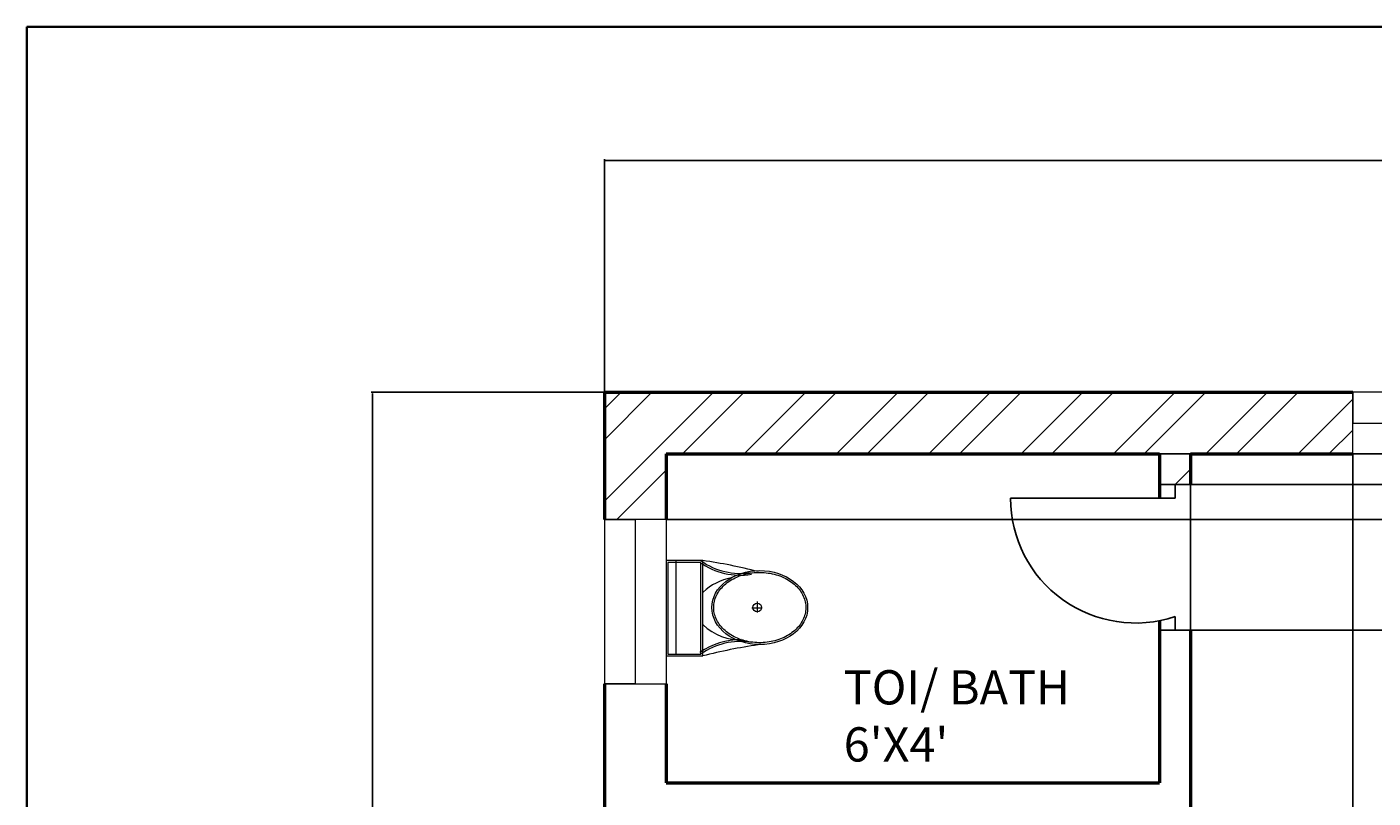
# Model space of a CAD drawing. Units: inches. Extents: x 2310 to 2937, y 1113 to 2410.
# Tile 18 of 23: x 2310 to 2507, y 2297 to 2410. Entities that reach past the tile are written whole.
import ezdxf

# ---------------------------------------------------------------- set-up
doc = ezdxf.new("R2010")
doc.units = ezdxf.units.IN
for name, color, linetype, lineweight in [('A-ANNO-DIMS', 2, 'Continuous', 18), ('A-ANNO-TTLB', 7, 'Continuous', 35), ('A-AREA-IDEN', 7, 'Continuous', 18), ('A-DOOR', 31, 'Continuous', 25), ('A-FLOR-FIXT', 9, 'Continuous', 18), ('A-GLAZ', 191, 'Continuous', 20), ('A-WALL', 7, 'Continuous', 50), ('A-WALL-PATT', 85, 'Continuous', 13)]:
    doc.layers.add(name, color=color, linetype=linetype, lineweight=lineweight)
doc.styles.get("Standard").update_dxf_attribs({"font": 'arial.ttf'})
doc.dimstyles.get("Standard").update_dxf_attribs({"dimtxt": 0.18, "dimasz": 0.18, "dimexe": 0.18, "dimexo": 0.0625, "dimgap": 0.09, "dimtad": 0, "dimtih": 1, "dimtoh": 1, "dimdec": 4, "dimzin": 0, "dimdsep": 46, "dimtxsty": 'Standard', "dimcen": 0.09, "dimadec": 0, "dimazin": 0, "dimtfac": 1, "dimtdec": 4, "dimtofl": 0, "dimtmove": 0, "dimatfit": 3, "dimfxl": 1, "dimtolj": 1, "dimtzin": 0, "dimarcsym": 0})

# ---------------------------------------------------------------- blocks, each defined once
blk = doc.blocks.new('A$C31115884')
for p, q in [((257.5, 466.4), (257.5, 523.2)), ((283.1, 497.7), (223.4, 497.7)), ((0, 200), (0, 0)), ((520, 200), (0, 200)), ((10, 190), (10, 10)), ((510, 190), (10, 190)), ((510, 10), (510, 190)), ((520, 0), (520, 200)), ((510, 54.5), (0, 54.5)), ((10, 10), (510, 10)), ((0, 0), (520, 0))]:
    blk.add_line(p, q)
blk.add_circle((255.6, 496.4), 23.6)
for centre, radius, start, end in [((2777.7, -204.6), 2807, 165.4549, 171.71327), ((-294.5, 403.3), 364.7, 324.20913, 9.34987), ((-294.5, 403.3), 374.7, 324.20913, 9.34987), ((805.8, 403.3), 364.7, 170.65013, 215.79087), ((3237, 905), 2807, 188.28673, 194.5451), ((139.5, 406.2), 293.5, 315.84364, 2.65635), ((805.8, 403.3), 374.7, 179.20365, 215.79087), ((383.6, 406.2), 293.5, 190.27735, 224.15636)]:
    blk.add_arc(centre, radius, start, end)
blk.add_ellipse((256.2, 509.9), major_axis=(0, -260.7), ratio=0.772727)
blk.add_open_spline([(256.2, 259.2), (263.1, 259.2), (270, 259.7), (287.8, 262.3), (298.7, 265.1), (319.9, 273.1), (330.2, 278.4), (350.1, 291.1), (359.7, 298.7), (377.7, 315.9), (386.2, 325.5), (401.7, 346.6), (408.8, 358.1), (421.3, 382.5), (426.8, 395.5), (435.9, 422.4), (439.5, 436.4), (444.8, 465.1), (446.5, 479.7), (447.9, 509.2), (447.6, 524), (445, 553.3), (442.7, 567.8), (436.3, 596), (432.1, 609.7), (421.9, 636), (416, 648.6), (402.5, 672.1), (395, 683), (378.6, 703), (369.8, 712.1), (351.1, 728), (341.3, 734.8), (320.9, 746.2), (310.4, 750.7), (288.9, 757.3), (278, 759.4), (256, 761), (245, 760.6), (223.1, 757.2), (212.3, 754.3), (191.1, 746.1), (180.8, 740.7), (160.9, 727.8), (151.4, 720.1), (133.5, 702.7), (125.1, 693), (109.6, 671.7), (102.6, 660.2), (90.2, 635.7), (84.9, 622.7), (76, 595.6), (72.4, 581.6), (67.2, 552.9), (65.6, 538.2), (64.4, 508.8), (64.8, 494), (67.5, 464.7), (69.9, 450.2), (76.6, 422), (80.8, 408.3), (91.1, 382.2), (97.2, 369.7), (110.8, 346.3), (118.4, 335.4), (134.8, 315.6), (143.7, 306.7), (162.4, 290.9), (172.3, 284.2), (192.8, 273), (203.3, 268.6), (224.8, 262.2), (235.8, 260.2), (249.9, 259.3), (253, 259.2), (256.2, 259.2)], degree=3, knots=[0, 0, 0, 0, 0.110105, 0.110105, 0.285049, 0.285049, 0.459994, 0.459994, 0.634938, 0.634938, 0.809882, 0.809882, 0.984827, 0.984827, 1.159771, 1.159771, 1.334715, 1.334715, 1.50966, 1.50966, 1.684604, 1.684604, 1.859549, 1.859549, 2.034493, 2.034493, 2.209437, 2.209437, 2.384382, 2.384382, 2.559326, 2.559326, 2.73427, 2.73427, 2.909215, 2.909215, 3.084159, 3.084159, 3.259103, 3.259103, 3.434048, 3.434048, 3.608992, 3.608992, 3.783936, 3.783936, 3.958881, 3.958881, 4.133825, 4.133825, 4.30877, 4.30877, 4.483714, 4.483714, 4.658658, 4.658658, 4.833603, 4.833603, 5.008547, 5.008547, 5.183491, 5.183491, 5.358436, 5.358436, 5.53338, 5.53338, 5.708324, 5.708324, 5.883269, 5.883269, 6.058213, 6.058213, 6.233158, 6.233158, 6.283185, 6.283185, 6.283185, 6.283185])
blk = doc.blocks.new('WIN-60IN-HEAD')
for p, q in [((0, 0), (0, 9)), ((0, 9), (0, 4.5)), ((60, 9), (0, 9)), ((60, 4.5), (60, 9)), ((60, 9), (60, 0)), ((0, 4.5), (60, 4.5)), ((0, 0), (60, 0))]:
    blk.add_line(p, q)
blk = doc.blocks.new('*D39')
at = {"layer": 'A-ANNO-DIMS', "color": 0, "lineweight": -2, "transparency": 16777216}
for p, q in [((2394.49, 2356.58), (2394.49, 2390.54)), ((2394.67, 2390.36), (2608.84, 2390.36)), ((2823.81, 2390.36), (2609.63, 2390.36)), ((2823.99, 2356.58), (2823.99, 2390.54))]:
    blk.add_line(p, q, dxfattribs=at)
at = {"layer": 'A-ANNO-DIMS', "color": 0, "transparency": 16777216}
for points in [[(2394.67, 2390.39), (2394.67, 2390.33), (2394.49, 2390.36)], [(2823.81, 2390.39), (2823.81, 2390.33), (2823.99, 2390.36)]]:
    blk.add_solid(points, dxfattribs=at)
at = {"layer": 'Defpoints', "color": 0, "transparency": 16777216}
for p in [(2823.99, 2390.36), (2394.49, 2356.51), (2823.99, 2356.51)]:
    blk.add_point(p, dxfattribs=at)
at = {"layer": 'A-ANNO-DIMS', "color": 0, "transparency": 16777216, "insert": (2609.24, 2390.36), "char_height": 0.18, "attachment_point": 5}
blk.add_mtext('\\A1;429.5', dxfattribs=at)
blk = doc.blocks.new('*D40')
at = {"layer": 'A-ANNO-DIMS', "color": 0, "lineweight": -2, "transparency": 16777216}
for p, q in [((2394.42, 2356.51), (2360.46, 2356.51)), ((2360.64, 2356.33), (2360.64, 2046.7)), ((2360.64, 1736.69), (2360.64, 2046.33)), ((2394.42, 1736.51), (2360.46, 1736.51))]:
    blk.add_line(p, q, dxfattribs=at)
at = {"layer": 'A-ANNO-DIMS', "color": 0, "transparency": 16777216}
for points in [[(2360.61, 2356.33), (2360.67, 2356.33), (2360.64, 2356.51)], [(2360.61, 1736.69), (2360.67, 1736.69), (2360.64, 1736.51)]]:
    blk.add_solid(points, dxfattribs=at)
at = {"layer": 'Defpoints', "color": 0, "transparency": 16777216}
for p in [(2360.64, 2356.51), (2394.49, 2356.51), (2394.49, 1736.51)]:
    blk.add_point(p, dxfattribs=at)
at = {"layer": 'A-ANNO-DIMS', "color": 0, "transparency": 16777216, "insert": (2360.64, 2046.51), "char_height": 0.18, "attachment_point": 5}
blk.add_mtext('\\A1;620', dxfattribs=at)
blk = doc.blocks.new('*D41')
at = {"layer": 'A-ANNO-DIMS', "color": 0, "lineweight": -2, "transparency": 16777216}
for p, q in [((2479.99, 2347.45), (2479.99, 1649.5)), ((2503.66, 2347.45), (2503.66, 1649.5)), ((2480.17, 1649.68), (2491.36, 1649.68)), ((2503.48, 1649.68), (2492.29, 1649.68))]:
    blk.add_line(p, q, dxfattribs=at)
at = {"layer": 'A-ANNO-DIMS', "color": 0, "transparency": 16777216}
for points in [[(2480.17, 1649.71), (2480.17, 1649.65), (2479.99, 1649.68)], [(2503.48, 1649.71), (2503.48, 1649.65), (2503.66, 1649.68)]]:
    blk.add_solid(points, dxfattribs=at)
at = {"layer": 'Defpoints', "color": 0, "transparency": 16777216}
for p in [(2479.99, 2347.51), (2503.66, 2347.51), (2503.66, 1649.68)]:
    blk.add_point(p, dxfattribs=at)
at = {"layer": 'A-ANNO-DIMS', "color": 0, "transparency": 16777216, "insert": (2491.82, 1649.68), "char_height": 0.18, "attachment_point": 5}
blk.add_mtext('\\A1;23.676', dxfattribs=at)
blk = doc.blocks.new('*D52')
at = {"layer": 'A-ANNO-DIMS', "color": 0, "lineweight": -2, "transparency": 16777216}
for p, q in [((2403.55, 2347.51), (2858.02, 2347.51)), ((2857.84, 2347.33), (2857.84, 2342.9)), ((2857.84, 2338.1), (2857.84, 2342.54)), ((2403.55, 2337.92), (2858.02, 2337.92))]:
    blk.add_line(p, q, dxfattribs=at)
at = {"layer": 'A-ANNO-DIMS', "color": 0, "transparency": 16777216}
for points in [[(2857.81, 2347.33), (2857.87, 2347.33), (2857.84, 2347.51)], [(2857.81, 2338.1), (2857.87, 2338.1), (2857.84, 2337.92)]]:
    blk.add_solid(points, dxfattribs=at)
at = {"layer": 'Defpoints', "color": 0, "transparency": 16777216}
for p in [(2403.49, 2347.51), (2403.49, 2337.92), (2857.84, 2337.92)]:
    blk.add_point(p, dxfattribs=at)
at = {"layer": 'A-ANNO-DIMS', "color": 0, "transparency": 16777216, "insert": (2857.84, 2342.72), "char_height": 0.18, "attachment_point": 5}
blk.add_mtext('\\A1;9.59', dxfattribs=at)
blk = doc.blocks.new('*D59')
at = {"layer": 'A-ANNO-DIMS', "color": 0, "lineweight": -2, "transparency": 16777216}
for p, q in [((2480.05, 2343.04), (2858.02, 2343.04)), ((2857.84, 2342.86), (2857.84, 2332.58)), ((2857.84, 2321.94), (2857.84, 2332.22)), ((2480.05, 2321.76), (2858.02, 2321.76))]:
    blk.add_line(p, q, dxfattribs=at)
at = {"layer": 'A-ANNO-DIMS', "color": 0, "transparency": 16777216}
for points in [[(2857.81, 2342.86), (2857.87, 2342.86), (2857.84, 2343.04)], [(2857.81, 2321.94), (2857.87, 2321.94), (2857.84, 2321.76)]]:
    blk.add_solid(points, dxfattribs=at)
at = {"layer": 'Defpoints', "color": 0, "transparency": 16777216}
for p in [(2479.99, 2343.04), (2857.84, 2343.04), (2479.99, 2321.76)]:
    blk.add_point(p, dxfattribs=at)
at = {"layer": 'A-ANNO-DIMS', "color": 0, "transparency": 16777216, "insert": (2857.84, 2332.4), "char_height": 0.18, "attachment_point": 5}
blk.add_mtext('\\A1;21.28', dxfattribs=at)

msp = doc.modelspace()

# ---------------------------------------------------------------- hatches: boundary and pattern name
at = {"layer": 'A-WALL-PATT'}
h = msp.add_hatch(dxfattribs=at)
h.set_pattern_fill('ANSI32', color=256)
h.paths.add_polyline_path([(2639.1394, 2356.5139), (2563.662, 2356.5139), (2563.662, 2347.5139), (2606.9859, 2347.5139), (2606.9859, 2210.5139), (2514.2692, 2210.5139), (2514.2692, 2206.0139), (2606.9859, 2206.0139), (2606.9859, 2098.0139), (2602.689, 2098.0139), (2602.689, 2093.5139), (2615.5262, 2093.5139), (2615.5262, 2095.7639), (2615.5262, 2098.0139), (2611.4859, 2098.0139), (2611.4859, 2206.0139), (2703.9391, 2206.0139), (2703.9391, 2208.2639), (2703.9391, 2210.5139), (2611.4859, 2210.5139), (2611.4859, 2347.5139), (2639.1394, 2347.5139)])
h.paths.add_polyline_path([(2823.9859, 2356.5139), (2699.1394, 2356.5139), (2699.1394, 2347.5139), (2738.4859, 2347.5139), (2738.4859, 2343.9266), (2742.9859, 2343.9266), (2742.9859, 2347.5139), (2814.9859, 2347.5139), (2814.9859, 2336.76), (2823.9859, 2336.76)])
h.paths.add_polyline_path([(2823.9859, 2312.76), (2814.9859, 2312.76), (2814.9859, 2299.5139), (2742.9859, 2299.5139), (2742.9859, 2323.0159), (2740.7359, 2323.0159), (2738.4859, 2323.0159), (2738.4859, 2210.5139), (2734.5483, 2210.5139), (2734.5483, 2206.0139), (2746.8769, 2206.0139), (2746.8769, 2208.2639), (2746.8769, 2210.5139), (2742.9859, 2210.5139), (2742.9859, 2295.0139), (2814.9859, 2295.0139), (2814.9859, 2269.8977), (2823.9859, 2269.8977)])
h.paths.add_polyline_path([(2823.9859, 2210.5139), (2823.9859, 2233.8977), (2819.4859, 2233.8977), (2814.9859, 2233.8977), (2814.9859, 2210.5139), (2769.9745, 2210.5139), (2769.9745, 2206.0139), (2814.9859, 2206.0139), (2814.9859, 2178.3027), (2823.9859, 2178.3027)])
h.paths.add_polyline_path([(2823.9859, 2118.3027), (2819.4859, 2118.3027), (2814.9859, 2118.3027), (2814.9859, 2098.0139), (2647.0333, 2098.0139), (2647.0333, 2093.5139), (2814.9859, 2093.5139), (2814.9859, 1999.5139), (2650.6052, 1999.5139), (2650.6052, 1995.0139), (2814.9859, 1995.0139), (2814.9859, 1969.9784), (2823.9859, 1969.9784)])
h.paths.add_polyline_path([(2403.4859, 2093.5139), (2569.9888, 2093.5139), (2569.9888, 2095.7639), (2569.9888, 2098.0139), (2403.4859, 2098.0139), (2403.4859, 2131.7587), (2394.4859, 2131.7587), (2394.4859, 1967.522), (2403.4859, 1967.522), (2403.4859, 1995.0139), (2569.8903, 1995.0139), (2569.8903, 1997.2639), (2569.8903, 1999.5139), (2403.4859, 1999.5139)])
h.paths.add_polyline_path([(2503.662, 2356.5139), (2394.4859, 2356.5139), (2394.4859, 2337.9231), (2398.9859, 2337.9231), (2403.4859, 2337.9231), (2403.4859, 2347.5139), (2475.4859, 2347.5139), (2475.4859, 2343.0384), (2479.9859, 2343.0384), (2479.9859, 2347.5139), (2503.662, 2347.5139)])
h.paths.add_polyline_path([(2498.3065, 1745.5139), (2479.9859, 1745.5139), (2479.9859, 1749.1663), (2477.7359, 1749.1663), (2475.4859, 1749.1663), (2475.4859, 1745.5139), (2403.4859, 1745.5139), (2403.4859, 1753.6409), (2398.9859, 1753.6409), (2394.4859, 1753.6409), (2394.4859, 1736.5139), (2498.3065, 1736.5139), (2498.3065, 1741.0139)])
h.paths.add_polyline_path([(2479.9859, 1882.5139), (2483.9367, 1882.5139), (2483.9367, 1887.0139), (2471.5501, 1887.0139), (2471.5501, 1885.1969), (2471.5501, 1882.5139), (2475.4859, 1882.5139), (2475.4859, 1798.0139), (2403.4859, 1798.0139), (2403.4859, 1828.0433), (2402.2852, 1828.0433), (2394.4859, 1828.0433), (2394.4859, 1777.6409), (2403.4859, 1777.6409), (2403.4859, 1793.5139), (2475.4859, 1793.5139), (2475.4859, 1769.1696), (2479.9859, 1769.1696)])
h.paths.add_polyline_path([(2403.4859, 1907.522), (2398.9859, 1907.522), (2394.4859, 1907.522), (2394.4859, 1864.0433), (2403.4859, 1864.0433), (2403.4859, 1882.5139), (2448.9325, 1882.5139), (2448.9325, 1884.7639), (2448.9325, 1887.0139), (2403.4859, 1887.0139)])
h.paths.add_polyline_path([(2702.2061, 1887.0139), (2611.4859, 1887.0139), (2611.4859, 1995.0139), (2615.6132, 1995.0139), (2615.6132, 1999.5139), (2602.4798, 1999.5139), (2602.4798, 1997.2639), (2602.4798, 1995.0139), (2606.9859, 1995.0139), (2606.9859, 1887.0139), (2516.2443, 1887.0139), (2516.2443, 1884.7639), (2516.2443, 1882.5139), (2606.9859, 1882.5139), (2606.9859, 1745.5139), (2558.3065, 1745.5139), (2558.3065, 1736.5139), (2638.8921, 1736.5139), (2638.8921, 1741.0139), (2638.8921, 1745.5139), (2611.4859, 1745.5139), (2611.4859, 1882.5139), (2702.2061, 1882.5139)])
h.paths.add_polyline_path([(2823.9859, 1909.9784), (2819.4859, 1909.9784), (2814.9859, 1909.9784), (2814.9859, 1887.0139), (2769.144, 1887.0139), (2769.144, 1884.7639), (2769.144, 1882.5139), (2814.9859, 1882.5139), (2814.9859, 1854.1704), (2823.9859, 1854.1704)])
h.paths.add_polyline_path([(2823.9859, 1818.1704), (2819.4859, 1818.1704), (2814.9859, 1818.1704), (2814.9859, 1798.0139), (2742.9859, 1798.0139), (2742.9859, 1882.5139), (2746.805, 1882.5139), (2746.805, 1887.0139), (2733.7334, 1887.0139), (2733.7334, 1884.7639), (2733.7334, 1882.5139), (2738.4859, 1882.5139), (2738.4859, 1771.1728), (2740.7359, 1771.1728), (2742.9859, 1771.1728), (2742.9859, 1793.5139), (2814.9859, 1793.5139), (2814.9859, 1783.6684), (2823.9859, 1783.6684)])
h.paths.add_polyline_path([(2823.9859, 1759.6684), (2814.9859, 1759.6684), (2814.9859, 1745.5139), (2742.9859, 1745.5139), (2742.9859, 1748.9831), (2740.7359, 1748.9831), (2738.4859, 1748.9831), (2738.4859, 1745.5139), (2698.8921, 1745.5139), (2698.8921, 1736.5139), (2823.9859, 1736.5139)])

# ---------------------------------------------------------------- linework, layer by layer
at = {"layer": 'A-ANNO-TTLB'}
msp.add_lwpolyline([(2310.2498, 2409.8427), (2937.0534, 2409.8427), (2937.0534, 1616.036), (2310.2498, 1616.036)], close=True, dxfattribs=at)
at = {"layer": 'A-DOOR'}
for p, q in [((2475.4859, 2343.0384), (2479.9859, 2343.0384)), ((2479.9859, 2343.0384), (2477.7359, 2343.0384)), ((2477.7359, 2343.0384), (2477.7359, 2341.0384)), ((2477.7359, 2341.0384), (2453.7359, 2341.0384)), ((2477.7359, 2321.7598), (2477.7359, 2323.7598)), ((2475.4859, 2321.7598), (2479.9859, 2321.7598)), ((2479.9859, 2321.7598), (2477.7359, 2321.7598))]:
    msp.add_line(p, q, dxfattribs=at)
msp.add_arc((2471.9557, 2341.0384), 18.2198, 180, 288.496755, dxfattribs=at)
at = {"layer": 'A-GLAZ'}
for p, q in [((2503.662, 2356.5139), (2503.662, 2356.5139)), ((2403.4859, 2337.9231), (2394.4859, 2337.9231)), ((2394.4859, 2337.9231), (2398.9859, 2337.9231)), ((2394.4859, 2337.9231), (2394.4859, 2337.9231)), ((2394.4859, 2337.9231), (2394.4859, 2313.9231)), ((2398.9859, 2337.9231), (2398.9859, 2313.9231)), ((2403.4859, 2337.9231), (2403.4859, 2337.9231)), ((2403.4859, 2337.9231), (2403.4859, 2313.9231)), ((2398.9859, 2313.9231), (2394.4859, 2313.9231)), ((2394.4859, 2313.9231), (2403.4859, 2313.9231)), ((2403.4859, 2313.9231), (2403.4859, 2313.9231))]:
    msp.add_line(p, q, dxfattribs=at)
at = {"layer": 'A-WALL'}
for p, q in [((2394.4859, 2356.5139), (2503.662, 2356.5139)), ((2394.4859, 2356.5139), (2394.4859, 2337.9231)), ((2403.4859, 2347.5139), (2475.4859, 2347.5139)), ((2403.4859, 2347.5139), (2403.4859, 2337.9231)), ((2475.4859, 2347.5139), (2475.4859, 2341.0384)), ((2479.9859, 2347.5139), (2479.9859, 2343.0384)), ((2479.9859, 2347.5139), (2503.662, 2347.5139)), ((2475.4859, 2323.1639), (2475.4859, 2299.5139)), ((2479.9859, 2321.7598), (2479.9859, 2210.5139)), ((2394.4859, 2313.9231), (2394.4859, 2280.3697)), ((2403.4859, 2313.9231), (2403.4859, 2299.5139)), ((2403.4859, 2299.5139), (2475.4859, 2299.5139))]:
    msp.add_line(p, q, dxfattribs=at)

# ---------------------------------------------------------------- block references
at = {"layer": 'A-FLOR-FIXT', "xscale": 0.0268011493576733, "yscale": 0.0268011493576733, "zscale": 0.0268011493576733, "rotation": 270}
msp.add_blockref('A$C31115884', (2403.4859, 2331.9468), dxfattribs=at)
at = {"layer": 'A-GLAZ'}
msp.add_blockref('WIN-60IN-HEAD', (2503.662, 2347.5139), dxfattribs=at)

# ---------------------------------------------------------------- texts
at = {"layer": 'A-AREA-IDEN', "insert": (2429.3979, 2315.9354), "char_height": 5, "attachment_point": 1}
msp.add_mtext_dynamic_manual_height_columns("TOI/ BATH\\P6'X4'", width=269.662763, gutter_width=12.5, heights=[0], dxfattribs=at)

# ---------------------------------------------------------------- dimensions: what is measured, and where the dimension line sits
at = {"layer": 'A-ANNO-DIMS'}
for base, p1, p2, override, picture, middle in [((2823.9859, 2390.3639), (2394.4859, 2356.5139), (2823.9859, 2356.5139), {"dimdec": 1, "dimlfac": 1, "dimrnd": 0, "dimzin": 0, "dimdsep": 46, "dimlunit": 2}, '*D39', (2609.2359, 2390.3639)), ((2503.662, 1649.6807), (2479.9859, 2347.5139), (2503.662, 2347.5139), {"dimdec": 3, "dimlfac": 1, "dimrnd": 0, "dimzin": 0, "dimdsep": 46, "dimlunit": 2}, '*D41', (2491.824, 1649.6807))]:
    dim = msp.add_linear_dim(base=base, p1=p1, p2=p2, dimstyle='Standard', override=override, dxfattribs=at)
    dim.commit()
    dim.dimension.update_dxf_attribs({"geometry": picture, "text_midpoint": middle})
for base, p1, p2, override, picture, middle in [((2360.6359, 2356.5139), (2394.4859, 1736.5139), (2394.4859, 2356.5139), {"dimdec": 0, "dimlfac": 1, "dimrnd": 0, "dimzin": 0, "dimdsep": 46, "dimlunit": 2}, '*D40', (2360.6359, 2046.5139)), ((2857.8359, 2337.9231), (2403.4859, 2347.5139), (2403.4859, 2337.9231), {"dimdec": 2, "dimlfac": 1, "dimrnd": 0, "dimzin": 0, "dimdsep": 46, "dimlunit": 2}, '*D52', (2857.8359, 2342.7185)), ((2857.8359, 2343.0384), (2479.9859, 2321.7598), (2479.9859, 2343.0384), {"dimdec": 2, "dimlfac": 1, "dimrnd": 0, "dimzin": 0, "dimdsep": 46, "dimlunit": 2}, '*D59', (2857.8359, 2332.3991))]:
    dim = msp.add_linear_dim(base=base, p1=p1, p2=p2, angle=90, dimstyle='Standard', override=override, dxfattribs=at)
    dim.commit()
    dim.dimension.update_dxf_attribs({"geometry": picture, "text_midpoint": middle})

doc.saveas('drawing.dxf')
